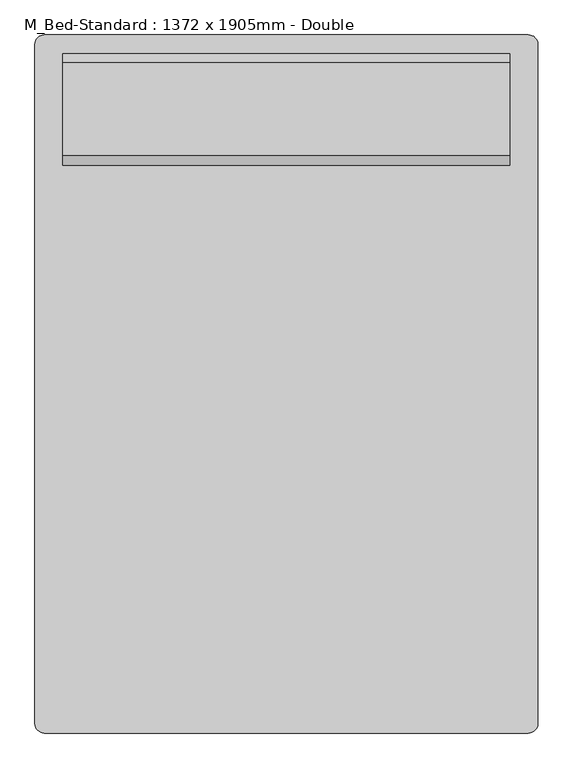
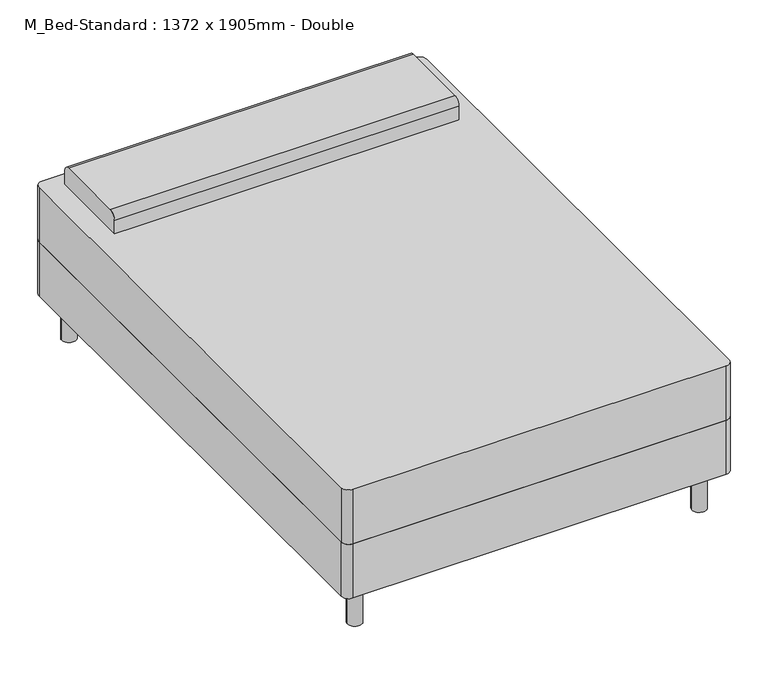
"""IFC4 building model written with IfcOpenShell, lengths in millimetres: furniture geometry, M_Bed-Standard : 1372 x 1905mm - Double."""

from ifc_helpers import new_model, si_unit, point, frame, frame_2d, origin, origin_with_axes, place, context, project, spatial, polyline, circle_curve, trimmed, segment, composite_curve, outline, extrude, source, transform, mapped, element, save


def m_bed_standard_1372_x_1905mm_double_64e02cd7(model_context):
    return source(origin(), model_context, "Body", "SweptSolid", [
        extrude(outline(composite_curve([segment(polyline([(-389.1114754, 906.904918), (932.0885246, 906.904918)]), True, "CONTINUOUS"), segment(trimmed(circle_curve(frame_2d((932.0885246, 881.504918)), 25.4), [point((932.0885246, 906.904918))], [point((957.4885246, 881.504918))], False, "CARTESIAN"), True, "CONTINUOUS"), segment(polyline([(957.4885246, 881.504918), (957.4885246, -972.695082)]), True, "CONTINUOUS"), segment(trimmed(circle_curve(frame_2d((932.0885246, -972.695082)), 25.4), [point((957.4885246, -972.695082))], [point((932.0885246, -998.095082))], False, "CARTESIAN"), True, "CONTINUOUS"), segment(polyline([(932.0885246, -998.095082), (-389.1114754, -998.095082)]), True, "CONTINUOUS"), segment(trimmed(circle_curve(frame_2d((-389.1114754, -972.695082)), 25.4), [point((-389.1114754, -998.095082))], [point((-414.5114754, -972.695082))], False, "CARTESIAN"), True, "CONTINUOUS"), segment(polyline([(-414.5114754, -972.695082), (-414.5114754, 881.504918)]), True, "CONTINUOUS"), segment(trimmed(circle_curve(frame_2d((-389.1114754, 881.504918)), 25.4), [point((-414.5114754, 881.504918))], [point((-389.1114754, 906.904918))], False, "CARTESIAN"), True, "CONTINUOUS")], self_intersect=False)), frame((0.0, 0.0, 355.6), z_axis=(0.0, 0.0, 1.0), x_axis=(1.0, 0.0, 0.0)), (0.0, 0.0, 1.0), 203.2),
        extrude(outline(composite_curve([segment(trimmed(circle_curve(frame_2d((-338.3114754, 830.704918)), 25.4), [point((-363.7114754, 830.704918))], [point((-312.9114754, 830.704918))], False, "CARTESIAN"), True, "CONTINUOUS"), segment(trimmed(circle_curve(frame_2d((-338.3114754, 830.704918)), 25.4), [point((-312.9114754, 830.704918))], [point((-363.7114754, 830.704918))], False, "CARTESIAN"), True, "CONTINUOUS")], self_intersect=False)), origin_with_axes(), (0.0, 0.0, 1.0), 152.4),
        extrude(outline(composite_curve([segment(trimmed(circle_curve(frame_2d((881.2885246, 830.704918)), 25.4), [point((855.8885246, 830.704918))], [point((906.6885246, 830.704918))], False, "CARTESIAN"), True, "CONTINUOUS"), segment(trimmed(circle_curve(frame_2d((881.2885246, 830.704918)), 25.4), [point((906.6885246, 830.704918))], [point((855.8885246, 830.704918))], False, "CARTESIAN"), True, "CONTINUOUS")], self_intersect=False)), origin_with_axes(), (0.0, 0.0, 1.0), 152.4),
        extrude(outline(composite_curve([segment(trimmed(circle_curve(frame_2d((881.2885246, -921.895082)), 25.4), [point((855.8885246, -921.895082))], [point((906.6885246, -921.895082))], False, "CARTESIAN"), True, "CONTINUOUS"), segment(trimmed(circle_curve(frame_2d((881.2885246, -921.895082)), 25.4), [point((906.6885246, -921.895082))], [point((855.8885246, -921.895082))], False, "CARTESIAN"), True, "CONTINUOUS")], self_intersect=False)), origin_with_axes(), (0.0, 0.0, 1.0), 152.4),
        extrude(outline(composite_curve([segment(trimmed(circle_curve(frame_2d((-338.3114754, -921.895082)), 25.4), [point((-363.7114754, -921.895082))], [point((-312.9114754, -921.895082))], False, "CARTESIAN"), True, "CONTINUOUS"), segment(trimmed(circle_curve(frame_2d((-338.3114754, -921.895082)), 25.4), [point((-312.9114754, -921.895082))], [point((-363.7114754, -921.895082))], False, "CARTESIAN"), True, "CONTINUOUS")], self_intersect=False)), origin_with_axes(), (0.0, 0.0, 1.0), 152.4),
        extrude(outline(composite_curve([segment(polyline([(551.304918, 558.8), (551.304918, 609.6)]), True, "CONTINUOUS"), segment(trimmed(circle_curve(frame_2d((576.704918, 609.6)), 25.4), [point((551.304918, 609.6))], [point((576.704918, 635.0))], False, "CARTESIAN"), True, "CONTINUOUS"), segment(polyline([(576.704918, 635.0), (830.704918, 635.0)]), True, "CONTINUOUS"), segment(trimmed(circle_curve(frame_2d((830.704918, 609.6)), 25.4), [point((830.704918, 635.0))], [point((856.104918, 609.6))], False, "CARTESIAN"), True, "CONTINUOUS"), segment(polyline([(856.104918, 609.6), (856.104918, 558.8), (551.304918, 558.8)]), True, "CONTINUOUS")], self_intersect=False)), frame((-338.3114754, 0.0, 0.0), z_axis=(1.0, 0.0, 0.0), x_axis=(0.0, 1.0, 0.0)), (0.0, 0.0, 1.0), 1219.6),
        extrude(outline(composite_curve([segment(polyline([(-414.5114754, -972.695082), (-414.5114754, 881.504918)]), True, "CONTINUOUS"), segment(trimmed(circle_curve(frame_2d((-389.1114754, 881.504918)), 25.4), [point((-414.5114754, 881.504918))], [point((-389.1114754, 906.904918))], False, "CARTESIAN"), True, "CONTINUOUS"), segment(polyline([(-389.1114754, 906.904918), (932.0885246, 906.904918)]), True, "CONTINUOUS"), segment(trimmed(circle_curve(frame_2d((932.0885246, 881.504918)), 25.4), [point((932.0885246, 906.904918))], [point((957.4885246, 881.504918))], False, "CARTESIAN"), True, "CONTINUOUS"), segment(polyline([(957.4885246, 881.504918), (957.4885246, -972.695082)]), True, "CONTINUOUS"), segment(trimmed(circle_curve(frame_2d((932.0885246, -972.695082)), 25.4), [point((957.4885246, -972.695082))], [point((932.0885246, -998.095082))], False, "CARTESIAN"), True, "CONTINUOUS"), segment(polyline([(932.0885246, -998.095082), (-389.1114754, -998.095082)]), True, "CONTINUOUS"), segment(trimmed(circle_curve(frame_2d((-389.1114754, -972.695082)), 25.4), [point((-389.1114754, -998.095082))], [point((-414.5114754, -972.695082))], False, "CARTESIAN"), True, "CONTINUOUS")], self_intersect=False)), frame((0.0, 0.0, 152.4), z_axis=(0.0, 0.0, 1.0), x_axis=(1.0, 0.0, 0.0)), (0.0, 0.0, 1.0), 203.2),
    ])


if __name__ == "__main__":
    model = new_model("IFC4")
    model_context = context("Model", 3, world=origin())
    ifc_project = project(units=[si_unit("LENGTHUNIT", "METRE", prefix="MILLI")], contexts=[model_context])
    site = spatial("IfcSite", under=ifc_project)
    building = spatial("IfcBuilding", under=site)
    placement = place(None, origin())
    m_bed_standard_1372_x_1905mm_double_shape = m_bed_standard_1372_x_1905mm_double_64e02cd7(model_context)
    element("IfcFurniture", 1, ObjectType="M_Bed-Standard : 1372 x 1905mm - Double", at=placement, inside=building, context=model_context, shape_type="MappedRepresentation", body=[
        mapped(m_bed_standard_1372_x_1905mm_double_shape, transform((0.0, 0.0, 0.0), x_axis=(1.0, 0.0, 0.0), y_axis=(0.0, 1.0, 0.0), z_axis=(0.0, 0.0, 1.0))),
    ])
    save(model, "model.ifc")

# Revit data of these elements
# Type "M_Bed-Standard : 1372 x 1905mm - Double"
#   Length = 6.25 ft
#   Width = 4.501312 ft
#   Leg Material = Steel, Chrome Plated
#   Mattress Material = Linen, White
#   Default Elevation = 0
# Element 1 (IfcFurniture, "M_Bed-Standard : 1372 x 1905mm - Double")
#   Materials on its faces: "Linen, White", "Steel, Chrome Plated"
# Materials
#   "Steel, Chrome Plated": class "Metal", colour RGB 17 17 17, transparency 0, Description = "Chromiuim plated steel", Cost = 0
#   "Linen, White": class "Textile", colour RGB 247 247 239, transparency 0, Description = "Linen, white", Cost = 0
